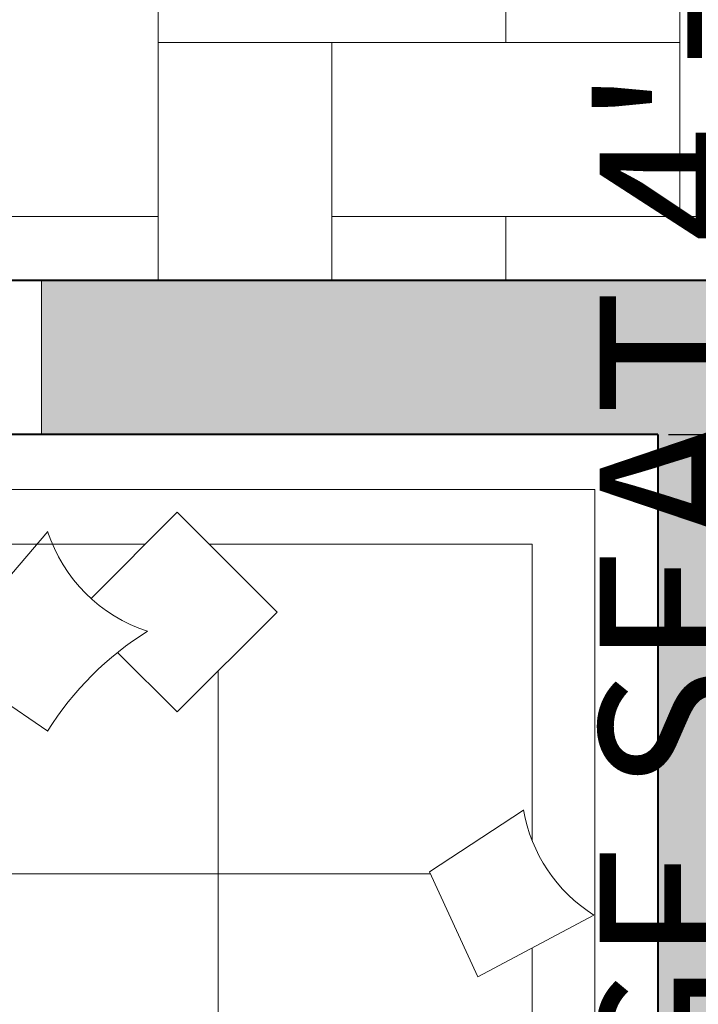
# Model space of a CAD drawing. Units: inches. Extents: x 2337 to 3570, y 1258 to 1938.
# Tile 15 of 30: x 2827 to 2866, y 1722 to 1779. Entities that reach past the tile are written whole.
import ezdxf

# ---------------------------------------------------------------- set-up
doc = ezdxf.new("R2010")
doc.units = ezdxf.units.IN
for name, color, linetype, lineweight in [('A-ANNO-DIMS', 2, 'Continuous', 18), ('A-FLOR-PATT', 252, 'Continuous', 13), ('A-GLAZ', 4, 'Continuous', 18), ('A-WALL', 7, 'Continuous', 40), ('furn', 8, 'Continuous', 18)]:
    doc.layers.add(name, color=color, linetype=linetype, lineweight=lineweight)
doc.layers.add('A-WALL-PATT', color=18, linetype='Continuous', lineweight=13, true_color=0x000000)
doc.styles.get("Standard").update_dxf_attribs({"font": 'arial.ttf'})
doc.dimstyles.new('ISO-25', dxfattribs={"dimtxt": 9, "dimasz": 2.5, "dimexe": 1.25, "dimexo": 0.625, "dimtad": 1, "dimdec": 1, "dimlunit": 3, "dimtxsty": 'Standard', "dimcen": 2.5, "dimadec": 0, "dimazin": 0, "dimtfac": 1, "dimtdec": 1, "dimtmove": 0, "dimatfit": 3, "dimfxl": 1, "dimarcsym": 0})

# ---------------------------------------------------------------- blocks, each defined once
blk = doc.blocks.new('sofa-11')
at = {"color": 0, "linetype": 'ByBlock'}
for p, q in [((0, 0), (0, 2.05)), ((0.1, 0.0875), (0.1, 1.95)), ((0.7, 1.9), (0.7, 0.3768)), ((0.2, 0.8184), (0.2, 1.8305)), ((0.2865, 0.8646), (0.1018, 0.766)), ((0.3637, 0.697), (0.2865, 0.8646)), ((0.2138, 0.5985), (0.3637, 0.697)), ((0.3623, 0.7), (2.6, 0.7)), ((0.2, 0.175), (0.2, 0.6475)), ((1.1431, 0.3556), (0.9718, 0.4727)), ((0.7655, 0.4423), (0.6064, 0.2832)), ((0.8605, 0.3474), (0.7655, 0.4423)), ((0.9718, 0.1545), (1.1431, 0.3556)), ((0.6064, 0.2832), (0.7655, 0.1241)), ((0.7655, 0.1241), (0.9027, 0.2613)), ((0.7147, 0.175), (0.2, 0.175)), ((1.5323, 0.175), (0.8164, 0.175)), ((0.1, 0.0875), (2.65, 0.0875)), ((2.775, 0), (0, 0))]:
    blk.add_line(p, q, dxfattribs=at)
for centre, radius, start, end in [((-0.0311, 0.556), 0.2485, 9.843, 57.6699), ((0.5496, 0.7358), 0.4975, 301.9301, 328.0699), ((0.7356, 0.0774), 0.2485, 18.0785, 71.9215)]:
    blk.add_arc(centre, radius, start, end, dxfattribs=at)
blk = doc.blocks.new('*D87')
at = {"layer": 'A-ANNO-DIMS', "color": 0, "lineweight": -2, "transparency": 16777216}
for p, q in [((2864.461, 1755.116), (2880.347, 1755.116)), ((2879.097, 1752.616), (2879.097, 1682.454)), ((2864.461, 1679.954), (2880.347, 1679.954))]:
    blk.add_line(p, q, dxfattribs=at)
at = {"layer": 'A-ANNO-DIMS', "color": 0, "transparency": 16777216}
for points in [[(2878.681, 1752.616), (2879.514, 1752.616), (2879.097, 1755.116)], [(2878.681, 1682.454), (2879.514, 1682.454), (2879.097, 1679.954)]]:
    blk.add_solid(points, dxfattribs=at)
at = {"layer": 'Defpoints', "color": 0, "transparency": 16777216}
for p in [(2863.836, 1755.116), (2863.836, 1679.954), (2879.097, 1679.954)]:
    blk.add_point(p, dxfattribs=at)
at = {"layer": 'A-ANNO-DIMS', "color": 0, "transparency": 16777216, "insert": (2873.874, 1717.535), "char_height": 9, "attachment_point": 5, "rotation": 90}
blk.add_mtext('6\'-3"', dxfattribs=at)
blk = doc.blocks.new('*D90')
at = {"layer": 'A-ANNO-DIMS', "color": 0, "lineweight": -2, "transparency": 16777216}
for p, q in [((2871.382, 1676.497), (2871.382, 1796.695)), ((2864.515, 1676.497), (2872.632, 1676.497)), ((2871.382, 1629.048), (2871.382, 1673.997)), ((2864.515, 1626.548), (2872.632, 1626.548))]:
    blk.add_line(p, q, dxfattribs=at)
at = {"layer": 'A-ANNO-DIMS', "color": 0, "transparency": 16777216}
for points in [[(2870.966, 1673.997), (2871.799, 1673.997), (2871.382, 1676.497)], [(2870.966, 1629.048), (2871.799, 1629.048), (2871.382, 1626.548)]]:
    blk.add_solid(points, dxfattribs=at)
at = {"layer": 'Defpoints', "color": 0, "transparency": 16777216}
for p in [(2863.89, 1676.497), (2871.382, 1676.497), (2863.89, 1626.548)]:
    blk.add_point(p, dxfattribs=at)
at = {"layer": 'A-ANNO-DIMS', "color": 0, "transparency": 16777216, "insert": (2866.101, 1737.846), "char_height": 9, "attachment_point": 5, "rotation": 90}
blk.add_mtext('LOUNGE SEAT 4\'-2"', dxfattribs=at)

msp = doc.modelspace()

# ---------------------------------------------------------------- hatches: boundary and pattern name
at = {"layer": 'A-FLOR-PATT', "transparency": 33554687}
h = msp.add_hatch(dxfattribs=at)
h.set_pattern_fill('AR-HBONE', color=256, scale=0.1, angle=45)
h.paths.add_polyline_path([(2902.836, 1875.116), (2899.836, 1875.116), (2899.836, 1887.116), (2671.836, 1887.116), (2671.836, 1857.116), (2681.836, 1857.116), (2681.836, 1810.116), (2719.836, 1810.116), (2719.836, 1764.116), (2872.836, 1764.116), (2899.836, 1764.116), (2899.836, 1779.116), (2902.836, 1779.116)])
h.paths.add_polyline_path([(2854.179, 1832.557), (2857.321, 1832.422), (2861.942, 1831.206, -0.088302), (2868.629, 1828.111), (2871.77, 1825.918, -0.105467), (2873.266, 1824.315), (2874.966, 1823.992), (2877.339, 1822.551), (2875.419, 1827.303), (2873.36, 1826.955, -0.132795), (2873.22, 1833.505), (2876.098, 1833.321), (2876.098, 1832.971), (2877.275, 1832.476, -0.091085), (2878.864, 1831.436, -0.069602), (2881.45, 1828.175, -0.141553), (2886.249, 1809.409, -0.141553), (2881.487, 1790.635, -0.069602), (2878.907, 1787.369, -0.091085), (2877.321, 1786.326), (2876.14, 1785.827, -0.354729), (2875.735, 1785.451), (2873.268, 1785.288, -0.132795), (2873.395, 1791.839), (2875.455, 1791.495), (2877.365, 1796.25), (2874.995, 1794.805), (2873.296, 1794.479, -0.105467), (2871.802, 1792.873), (2868.666, 1790.673, -0.088302), (2861.985, 1787.565), (2857.366, 1786.339), (2854.225, 1786.199), (2827.803, 1783.011, -0.315912), (2819.634, 1782.954), (2793.542, 1785.741), (2798.79, 1786.943), (2825.847, 1785.283, 0.026512), (2832.53, 1785.227), (2857.366, 1786.339), (2861.985, 1787.565, 0.088302), (2868.666, 1790.673), (2871.802, 1792.873, 0.191215), (2873.932, 1796.114), (2875.792, 1805.131, 0.102572), (2875.784, 1813.667), (2873.906, 1822.681, 0.191215), (2871.77, 1825.918), (2868.629, 1828.111, 0.088302), (2861.942, 1831.206), (2857.321, 1832.422), (2832.483, 1833.486, 0.026512), (2825.799, 1833.417), (2798.745, 1831.704), (2793.496, 1832.895), (2819.582, 1835.733, -0.315912), (2827.751, 1835.692)], flags=16)
h.paths.add_polyline_path([(2862.34, 1826.572), (2867.3, 1825.996, -0.316515), (2870.308, 1823.311), (2872.444, 1814.149, -0.11452), (2872.453, 1804.643), (2870.336, 1795.477, -0.316515), (2867.333, 1792.786), (2862.374, 1792.2, -0.464922), (2861.397, 1793.116), (2861.861, 1801.965), (2861.836, 1809.385), (2861.846, 1816.806), (2861.365, 1825.654, -0.464922)], flags=16)
h.paths.add_polyline_path([(2821.293, 1791.09), (2807.573, 1791.499, -0.405226), (2805.023, 1794.123), (2805.023, 1794.121, 0.40508), (2807.573, 1791.499), (2821.293, 1791.09, 0.423258), (2823.999, 1793.719), (2823.999, 1793.719, -0.423258)], flags=16)
h.paths.add_polyline_path([(2879.429, 1814.798), (2881.737, 1813.816), (2882.582, 1811.673), (2882.717, 1809.406), (2882.586, 1807.139), (2881.746, 1804.994), (2879.439, 1804.008), (2880.042, 1807.699, 0.081616), (2880.039, 1811.108)], flags=0)
h.paths.add_polyline_path([(2796.957, 1829.715), (2796.14, 1815.428, 0.029076), (2796.152, 1803.213), (2796.997, 1788.928, -0.409057), (2796.19, 1788.002), (2791.055, 1787.607), (2785.763, 1792.935, -0.173254), (2784.26, 1796.136), (2783.472, 1804.33, -0.047466), (2783.462, 1814.286), (2784.234, 1822.482, -0.173254), (2785.73, 1825.686), (2791.012, 1831.024), (2796.148, 1830.639, -0.409057)], flags=16)
h.paths.add_polyline_path([(2750.344, 1835.795), (2750.012, 1834.37, 0.040009), (2748.771, 1826.064), (2748.631, 1824.022), (2750.526, 1825.239), (2756.614, 1827.237), (2771.951, 1829.419), (2781.401, 1831.049), (2780.099, 1822.888), (2779.438, 1814.328), (2779.144, 1809.304), (2779.447, 1804.281), (2780.126, 1795.721), (2781.444, 1787.563), (2771.99, 1789.174), (2756.65, 1791.337), (2750.557, 1793.323), (2748.66, 1794.536), (2748.804, 1792.494, 0.040009), (2750.062, 1784.191), (2750.396, 1782.767), (2745.899, 1784.642), (2744.102, 1788.129), (2743.099, 1791.925), (2741.068, 1802.995), (2740.859, 1809.271), (2741.055, 1815.548), (2743.065, 1826.622), (2744.061, 1830.421), (2745.851, 1833.911)], flags=16)
h.paths.add_polyline_path([(2761.183, 1831.202), (2754.851, 1829.51), (2754.556, 1830.832, -0.143032), (2754.62, 1831.812), (2755.053, 1833), (2761.169, 1831.713, -0.789416)], flags=16)
h.paths.add_polyline_path([(2761.226, 1787.381), (2754.89, 1789.061), (2754.599, 1787.738, 0.143032), (2754.665, 1786.758), (2755.1, 1785.571), (2761.213, 1786.87, 0.789416)], flags=16)
h.paths.add_polyline_path([(2689.028, 1816.171), (2701.274, 1816.171), (2701.274, 1823.798), (2689.028, 1823.798)], flags=24)
h.paths.add_polyline_path([(2755.384, 1858.953), (2808.715, 1858.953), (2808.715, 1885.073), (2755.384, 1885.073)], flags=24)
at = {"layer": 'A-WALL-PATT'}
h = msp.add_hatch(color=256, dxfattribs=at)
h.dxf.hatch_style = 1
h.paths.add_polyline_path([(2671.836, 1857.116), (2455.836, 1857.116), (2455.836, 1824.116), (2464.836, 1824.116), (2464.836, 1848.116), (2671.836, 1848.116)])
h.paths.add_polyline_path([(2566.836, 1764.116), (2464.836, 1764.116), (2464.836, 1788.116), (2455.836, 1788.116), (2455.836, 1743.116), (2464.836, 1743.116), (2464.836, 1755.116), (2566.836, 1755.116)])
h.paths.add_polyline_path([(2683.836, 1761.116), (2683.836, 1764.116), (2602.836, 1764.116), (2602.836, 1755.116), (2608.836, 1755.116), (2608.836, 1701.116), (2662.836, 1701.116), (2662.836, 1605.116), (2671.836, 1605.116), (2671.836, 1713.116), (2662.836, 1713.116), (2662.836, 1707.116), (2614.836, 1707.116), (2614.836, 1755.116), (2662.836, 1755.116), (2662.836, 1749.116), (2671.836, 1749.116), (2671.836, 1755.116), (2683.836, 1755.116)])
h.paths.add_polyline_path([(2464.836, 1707.116), (2455.836, 1707.116), (2455.836, 1617.116), (2464.836, 1617.116), (2464.836, 1635.116), (2506.836, 1635.116), (2506.836, 1641.116), (2464.836, 1641.116)])
h.paths.add_polyline_path([(2542.836, 1551.116), (2464.836, 1551.116), (2464.836, 1569.116), (2455.836, 1569.116), (2455.836, 1518.116), (2464.836, 1518.116), (2464.836, 1542.116), (2542.836, 1542.116)])
h.paths.add_polyline_path([(2464.836, 1482.116), (2455.836, 1482.116), (2455.836, 1410.116), (2464.836, 1410.116)])
h.paths.add_polyline_path([(2626.836, 1350.116), (2590.836, 1350.116), (2590.836, 1380.116), (2584.836, 1380.116), (2584.836, 1350.116), (2464.836, 1350.116), (2464.836, 1374.116), (2455.836, 1374.116), (2455.836, 1341.116), (2626.836, 1341.116)])
h.paths.add_polyline_path([(2662.836, 1416.116), (2686.836, 1416.116), (2686.836, 1422.116), (2590.836, 1422.116), (2590.836, 1542.116), (2680.836, 1542.116), (2680.836, 1551.116), (2671.836, 1551.116), (2671.836, 1557.116), (2662.836, 1557.116), (2662.836, 1551.116), (2578.836, 1551.116), (2578.836, 1542.116), (2584.836, 1542.116), (2584.836, 1410.116), (2590.836, 1410.116), (2590.836, 1416.116), (2656.836, 1416.116), (2656.836, 1350.116), (2650.836, 1350.116), (2650.836, 1341.116), (2731.836, 1341.116), (2731.836, 1362.116), (2722.836, 1362.116), (2722.836, 1350.116), (2662.836, 1350.116)])
h.paths.add_polyline_path([(2731.836, 1434.116), (2722.836, 1434.116), (2722.836, 1422.116), (2716.836, 1422.116), (2716.836, 1416.116), (2722.836, 1416.116), (2722.836, 1386.116), (2731.836, 1386.116)], flags=17)
h.paths.add_polyline_path([(2731.836, 1542.116), (2752.836, 1542.116), (2752.836, 1551.116), (2716.836, 1551.116), (2716.836, 1545.116), (2716.836, 1542.116), (2722.836, 1542.116), (2722.836, 1482.116), (2731.836, 1482.116)])
h.paths.add_polyline_path([(2809.836, 1551.116), (2788.836, 1551.116), (2788.836, 1542.116), (2809.836, 1542.116), (2809.836, 1548.116)])
h.paths.add_polyline_path([(2872.836, 1647.116), (2863.836, 1647.116), (2863.836, 1551.116), (2857.836, 1551.116), (2857.836, 1548.116), (2857.836, 1542.116), (2872.836, 1542.116)])
h.paths.add_polyline_path([(2872.836, 1764.116), (2827.836, 1764.116), (2827.836, 1755.116), (2863.836, 1755.116), (2863.836, 1719.116), (2872.836, 1719.116)])
h.paths.add_polyline_path([(2755.836, 1764.116), (2719.836, 1764.116), (2719.836, 1755.116), (2755.836, 1755.116)])

# ---------------------------------------------------------------- linework, layer by layer
at = {"layer": 'A-GLAZ'}
msp.add_line((2827.836, 1764.116), (2827.836, 1755.116), dxfattribs=at)
at = {"layer": 'A-WALL'}
for p, q in [((2872.836, 1764.116), (2719.836, 1764.116)), ((2863.836, 1755.116), (2719.836, 1755.116)), ((2863.836, 1755.116), (2863.836, 1551.116))]:
    msp.add_line(p, q, dxfattribs=at)

# ---------------------------------------------------------------- block references
at = {"layer": 'furn', "xscale": 36.66436083614781, "yscale": 36.66436083614781, "zscale": 36.66436083614781, "rotation": 180}
msp.add_blockref('sofa-11', (2863.836, 1755.116), dxfattribs=at)

# ---------------------------------------------------------------- dimensions: what is measured, and where the dimension line sits
at = {"layer": 'A-ANNO-DIMS'}
dim = msp.add_linear_dim(base=(2871.382, 1676.497), p1=(2863.89, 1626.548), p2=(2863.89, 1676.497), angle=90, text='LOUNGE SEAT <>', dimstyle='ISO-25', override={"dimdec": 1, "dimlfac": 1, "dimrnd": 0, "dimzin": 1, "dimdsep": 46, "dimlunit": 4, "dimfrac": 2}, dxfattribs=at)
dim.commit()
dim.dimension.update_dxf_attribs({"geometry": '*D90', "text_midpoint": (2866.101, 1737.846)})
dim = msp.add_linear_dim(base=(2879.097, 1679.954), p1=(2863.836, 1755.116), p2=(2863.836, 1679.954), angle=270, dimstyle='ISO-25', override={"dimdec": 1, "dimlfac": 1, "dimrnd": 0, "dimzin": 1, "dimdsep": 46, "dimlunit": 4, "dimfrac": 2}, dxfattribs=at)
dim.commit()
dim.dimension.update_dxf_attribs({"geometry": '*D87', "text_midpoint": (2873.874, 1717.535)})

doc.saveas('drawing.dxf')
